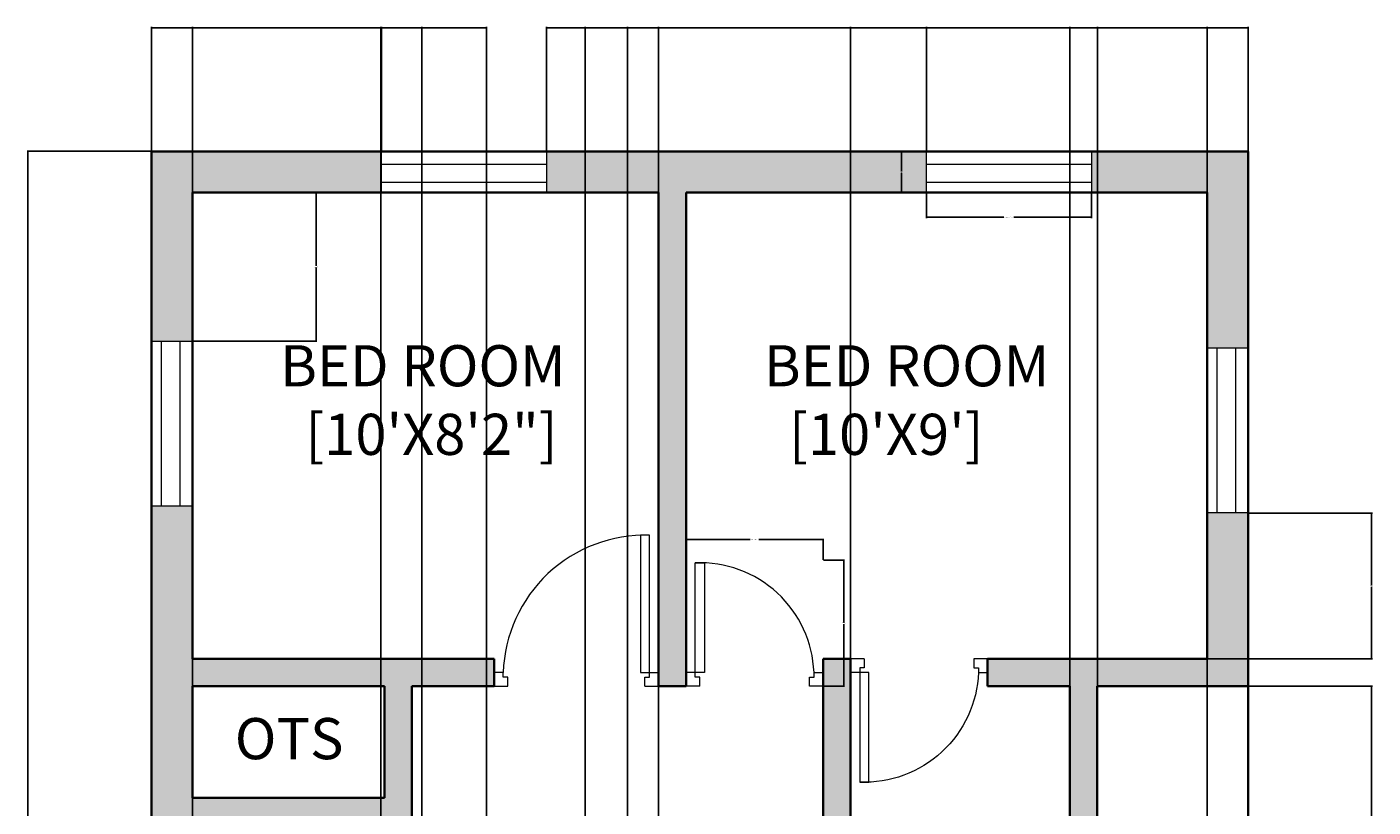
# Model space of a CAD drawing. Units: inches. Extents: x 1963 to 2258, y 1522 to 2116.
# Tile 3 of 3: x 1963 to 2257, y 1945 to 2116. Entities that reach past the tile are written whole.
import ezdxf

# ---------------------------------------------------------------- set-up
doc = ezdxf.new("R2010")
doc.units = ezdxf.units.IN
for name, color, linetype, lineweight in [('A-ANNO-DIMS', 2, 'Continuous', 18), ('A-AREA-IDEN', 7, 'Continuous', 18), ('A-DOOR', 3, 'Continuous', 18), ('A-GLAZ', 4, 'Continuous', 18), ('A-WALL', 7, 'Continuous', 35), ('A-WALL-PATT', 250, 'Continuous', 13)]:
    doc.layers.add(name, color=color, linetype=linetype, lineweight=lineweight)
doc.styles.get("Standard").update_dxf_attribs({"font": 'arial.ttf'})
doc.dimstyles.get("Standard").update_dxf_attribs({"dimtxt": 0.18, "dimasz": 0.18, "dimexe": 0.18, "dimexo": 0.0625, "dimgap": 0.09, "dimtad": 0, "dimtih": 1, "dimtoh": 1, "dimdec": 4, "dimzin": 0, "dimdsep": 46, "dimtxsty": 'Standard', "dimcen": 0.09, "dimadec": 0, "dimazin": 0, "dimtfac": 1, "dimtdec": 4, "dimtofl": 0, "dimtmove": 0, "dimatfit": 3, "dimfxl": 1, "dimtolj": 1, "dimtzin": 0, "dimarcsym": 0})

# ---------------------------------------------------------------- blocks, each defined once
blk = doc.blocks.new('WIN-36-9IN-WALL')
for p, q in [((-9, 0), (-9, 36.12)), ((-9, 36.12), (0, 36.12)), ((-6.81, 0), (-6.81, 36.12)), ((-4.5, 36.12), (-2.78, 36.12)), ((-2.78, 36.12), (-2.78, 0)), ((0, 36.12), (0, 0)), ((0, 0), (-9, 0)), ((-2.78, 0), (-6.81, 0)), ((0, 0), (-4.5, 0))]:
    blk.add_line(p, q)
blk = doc.blocks.new('DOOR-SWING-30IN')
for p, q in [((-3, -2), (-3, 0)), ((-3, 0), (0, 0)), ((-2, -2), (-3, -2)), ((-2, -3), (-2, -2)), ((0, 0), (0, -3)), ((0, 0), (0, -3)), ((0, -3), (-2, -3)), ((-27, -28), (-27, -26)), ((-27, -26), (-3, -26)), ((-3, -26), (-3, -28)), ((-3, -28), (-27, -28)), ((-2, -28), (-3, -28)), ((-3, -28), (-3, -30)), ((0, -27), (-2, -27)), ((-2, -27), (-2, -28)), ((0, -27), (0, -30)), ((-3, -30), (0, -30))]:
    blk.add_line(p, q)
blk.add_arc((-2, -27), 25.02, 92.2906, 182.2906)
blk = doc.blocks.new('DOOR-SWING-36IN')
for p, q in [((34, 33), (32, 33)), ((32, 33), (32, 3)), ((34, 3), (34, 33)), ((2, 3), (0, 3)), ((0, 3), (0, 0)), ((2, 2), (2, 3)), ((32, 3), (34, 3)), ((34, 2), (34, 3)), ((34, 3), (36, 3)), ((36, 3), (36, 0)), ((0, 0), (3, 0)), ((0, 0), (3, 0)), ((0, 0), (3, 0)), ((3, 2), (2, 2)), ((3, 0), (3, 2)), ((33, 0), (33, 2)), ((33, 2), (34, 2)), ((33, 0), (36, 0))]:
    blk.add_line(p, q)
blk.add_arc((33, 2), 31.02, 88.1524, 178.1524)
blk = doc.blocks.new('*D6')
at = {"layer": 'A-ANNO-DIMS', "color": 0, "lineweight": -2, "transparency": 16777216}
for p, q in [((2159.69, 2079.68), (2159.69, 2074.15)), ((2195.81, 2079.68), (2195.81, 2074.15)), ((2159.87, 2074.33), (2176.63, 2074.33)), ((2195.63, 2074.33), (2178.87, 2074.33))]:
    blk.add_line(p, q, dxfattribs=at)
at = {"layer": 'A-ANNO-DIMS', "color": 0, "transparency": 16777216}
for points in [[(2159.87, 2074.36), (2159.87, 2074.3), (2159.69, 2074.33)], [(2195.63, 2074.36), (2195.63, 2074.3), (2195.81, 2074.33)]]:
    blk.add_solid(points, dxfattribs=at)
at = {"layer": 'Defpoints', "color": 0, "transparency": 16777216}
for p in [(2159.69, 2079.75), (2195.81, 2079.75), (2159.69, 2074.33)]:
    blk.add_point(p, dxfattribs=at)
at = {"layer": 'A-ANNO-DIMS', "color": 0, "transparency": 16777216, "insert": (2177.75, 2074.33), "char_height": 0.18, "attachment_point": 5}
blk.add_mtext('\\A1;WINDOW 36 TYP.', dxfattribs=at)
blk = doc.blocks.new('*D7')
at = {"layer": 'A-ANNO-DIMS', "color": 0, "lineweight": -2, "transparency": 16777216}
for p, q in [((2159.63, 2088.75), (2154.09, 2088.75)), ((2154.27, 2088.57), (2154.27, 2084.43)), ((2154.27, 2079.93), (2154.27, 2084.07)), ((2159.63, 2079.75), (2154.09, 2079.75))]:
    blk.add_line(p, q, dxfattribs=at)
at = {"layer": 'A-ANNO-DIMS', "color": 0, "transparency": 16777216}
for points in [[(2154.24, 2088.57), (2154.3, 2088.57), (2154.27, 2088.75)], [(2154.24, 2079.93), (2154.3, 2079.93), (2154.27, 2079.75)]]:
    blk.add_solid(points, dxfattribs=at)
at = {"layer": 'Defpoints', "color": 0, "transparency": 16777216}
for p in [(2154.27, 2088.75), (2159.69, 2088.75), (2159.69, 2079.75)]:
    blk.add_point(p, dxfattribs=at)
at = {"layer": 'A-ANNO-DIMS', "color": 0, "transparency": 16777216, "insert": (2154.27, 2084.25), "char_height": 0.18, "attachment_point": 5}
blk.add_mtext('\\A1;9 TYP.', dxfattribs=at)
blk = doc.blocks.new('*D10')
at = {"layer": 'A-ANNO-DIMS', "color": 0, "lineweight": -2, "transparency": 16777216}
for p, q in [((2107.11, 1999.36), (2107.11, 2003.98)), ((2107.29, 2003.8), (2121.17, 2003.8)), ((2136.93, 2003.8), (2123.04, 2003.8)), ((2137.11, 1999.36), (2137.11, 2003.98))]:
    blk.add_line(p, q, dxfattribs=at)
at = {"layer": 'A-ANNO-DIMS', "color": 0, "transparency": 16777216}
for points in [[(2107.29, 2003.83), (2107.29, 2003.77), (2107.11, 2003.8)], [(2136.93, 2003.83), (2136.93, 2003.77), (2137.11, 2003.8)]]:
    blk.add_solid(points, dxfattribs=at)
at = {"layer": 'Defpoints', "color": 0, "transparency": 16777216}
for p in [(2137.11, 2003.8), (2107.11, 1999.3), (2137.11, 1999.3)]:
    blk.add_point(p, dxfattribs=at)
at = {"layer": 'A-ANNO-DIMS', "color": 0, "transparency": 16777216, "insert": (2122.11, 2003.8), "char_height": 0.18, "attachment_point": 5}
blk.add_mtext('\\A1;DOOR 30 TYP.', dxfattribs=at)
blk = doc.blocks.new('*D11')
at = {"layer": 'A-ANNO-DIMS', "color": 0, "lineweight": -2, "transparency": 16777216}
for p, q in [((2137.17, 1999.3), (2141.79, 1999.3)), ((2141.61, 1999.12), (2141.61, 1985.71)), ((2141.61, 1971.93), (2141.61, 1985.34)), ((2137.17, 1971.75), (2141.79, 1971.75))]:
    blk.add_line(p, q, dxfattribs=at)
at = {"layer": 'A-ANNO-DIMS', "color": 0, "transparency": 16777216}
for points in [[(2141.58, 1999.12), (2141.64, 1999.12), (2141.61, 1999.3)], [(2141.58, 1971.93), (2141.64, 1971.93), (2141.61, 1971.75)]]:
    blk.add_solid(points, dxfattribs=at)
at = {"layer": 'Defpoints', "color": 0, "transparency": 16777216}
for p in [(2137.11, 1999.3), (2137.11, 1971.75), (2141.61, 1971.75)]:
    blk.add_point(p, dxfattribs=at)
at = {"layer": 'A-ANNO-DIMS', "color": 0, "transparency": 16777216, "insert": (2141.61, 1985.52), "char_height": 0.18, "attachment_point": 5}
blk.add_mtext('\\A1;28 TYP.', dxfattribs=at)
blk = doc.blocks.new('*D15')
at = {"layer": 'A-ANNO-DIMS', "color": 0, "lineweight": -2, "transparency": 16777216}
for p, q in [((2094.32, 1548.81), (2094.32, 2115.96)), ((2094.5, 2115.78), (2157.26, 2115.78)), ((2220.93, 2115.78), (2158.17, 2115.78)), ((2221.11, 1548.81), (2221.11, 2115.96))]:
    blk.add_line(p, q, dxfattribs=at)
at = {"layer": 'A-ANNO-DIMS', "color": 0, "transparency": 16777216}
for points in [[(2094.5, 2115.81), (2094.5, 2115.75), (2094.32, 2115.78)], [(2220.93, 2115.81), (2220.93, 2115.75), (2221.11, 2115.78)]]:
    blk.add_solid(points, dxfattribs=at)
at = {"layer": 'Defpoints', "color": 0, "transparency": 16777216}
for p in [(2221.11, 2115.78), (2094.32, 1548.75), (2221.11, 1548.75)]:
    blk.add_point(p, dxfattribs=at)
at = {"layer": 'A-ANNO-DIMS', "color": 0, "transparency": 16777216, "insert": (2157.72, 2115.78), "char_height": 0.18, "attachment_point": 5}
blk.add_mtext('\\A1;126.79', dxfattribs=at)
blk = doc.blocks.new('*D16')
at = {"layer": 'A-ANNO-DIMS', "color": 0, "lineweight": -2, "transparency": 16777216}
for p, q in [((1990.11, 2088.81), (1990.11, 2115.96)), ((1990.29, 2115.78), (2014.88, 2115.78)), ((2040.25, 2115.78), (2015.66, 2115.78)), ((2040.43, 2088.81), (2040.43, 2115.96))]:
    blk.add_line(p, q, dxfattribs=at)
at = {"layer": 'A-ANNO-DIMS', "color": 0, "transparency": 16777216}
for points in [[(1990.29, 2115.81), (1990.29, 2115.75), (1990.11, 2115.78)], [(2040.25, 2115.81), (2040.25, 2115.75), (2040.43, 2115.78)]]:
    blk.add_solid(points, dxfattribs=at)
at = {"layer": 'Defpoints', "color": 0, "transparency": 16777216}
for p in [(2040.43, 2115.78), (1990.11, 2088.75), (2040.43, 2088.75)]:
    blk.add_point(p, dxfattribs=at)
at = {"layer": 'A-ANNO-DIMS', "color": 0, "transparency": 16777216, "insert": (2015.27, 2115.78), "char_height": 0.18, "attachment_point": 5}
blk.add_mtext('\\A1;50.32', dxfattribs=at)
blk = doc.blocks.new('*D17')
at = {"layer": 'A-ANNO-DIMS', "color": 0, "lineweight": -2, "transparency": 16777216}
for p, q in [((2076.55, 2088.81), (2076.55, 2115.96)), ((2076.73, 2115.78), (2117.73, 2115.78)), ((2159.51, 2115.78), (2118.51, 2115.78)), ((2159.69, 2088.81), (2159.69, 2115.96))]:
    blk.add_line(p, q, dxfattribs=at)
at = {"layer": 'A-ANNO-DIMS', "color": 0, "transparency": 16777216}
for points in [[(2076.73, 2115.81), (2076.73, 2115.75), (2076.55, 2115.78)], [(2159.51, 2115.81), (2159.51, 2115.75), (2159.69, 2115.78)]]:
    blk.add_solid(points, dxfattribs=at)
at = {"layer": 'Defpoints', "color": 0, "transparency": 16777216}
for p in [(2159.69, 2115.78), (2076.55, 2088.75), (2159.69, 2088.75)]:
    blk.add_point(p, dxfattribs=at)
at = {"layer": 'A-ANNO-DIMS', "color": 0, "transparency": 16777216, "insert": (2118.12, 2115.78), "char_height": 0.18, "attachment_point": 5}
blk.add_mtext('\\A1;83.14', dxfattribs=at)
blk = doc.blocks.new('*D18')
at = {"layer": 'A-ANNO-DIMS', "color": 0, "lineweight": -2, "transparency": 16777216}
for p, q in [((1999.11, 2079.68), (1999.11, 1521.53)), ((2101.11, 2079.68), (2101.11, 1521.53)), ((1999.29, 1521.71), (2049.83, 1521.71)), ((2100.93, 1521.71), (2050.39, 1521.71))]:
    blk.add_line(p, q, dxfattribs=at)
at = {"layer": 'A-ANNO-DIMS', "color": 0, "transparency": 16777216}
for points in [[(1999.29, 1521.74), (1999.29, 1521.68), (1999.11, 1521.71)], [(2100.93, 1521.74), (2100.93, 1521.68), (2101.11, 1521.71)]]:
    blk.add_solid(points, dxfattribs=at)
at = {"layer": 'Defpoints', "color": 0, "transparency": 16777216}
for p in [(1999.11, 2079.75), (2101.11, 2079.75), (2101.11, 1521.71)]:
    blk.add_point(p, dxfattribs=at)
at = {"layer": 'A-ANNO-DIMS', "color": 0, "transparency": 16777216, "insert": (2050.11, 1521.71), "char_height": 0.18, "attachment_point": 5}
blk.add_mtext('\\A1;102', dxfattribs=at)
blk = doc.blocks.new('*D25')
at = {"layer": 'A-ANNO-DIMS', "color": 0, "lineweight": -2, "transparency": 16777216}
for p, q in [((1999.17, 2079.75), (2026.32, 2079.75)), ((2026.14, 2079.57), (2026.14, 2063.67)), ((2026.14, 2047.42), (2026.14, 2063.31)), ((1999.17, 2047.24), (2026.32, 2047.24))]:
    blk.add_line(p, q, dxfattribs=at)
at = {"layer": 'A-ANNO-DIMS', "color": 0, "transparency": 16777216}
for points in [[(2026.11, 2079.57), (2026.17, 2079.57), (2026.14, 2079.75)], [(2026.11, 2047.42), (2026.17, 2047.42), (2026.14, 2047.24)]]:
    blk.add_solid(points, dxfattribs=at)
at = {"layer": 'Defpoints', "color": 0, "transparency": 16777216}
for p in [(1999.11, 2079.75), (1999.11, 2047.24), (2026.14, 2047.24)]:
    blk.add_point(p, dxfattribs=at)
at = {"layer": 'A-ANNO-DIMS', "color": 0, "transparency": 16777216, "insert": (2026.14, 2063.49), "char_height": 0.18, "attachment_point": 5}
blk.add_mtext('\\A1;32.51', dxfattribs=at)
blk = doc.blocks.new('*D29')
at = {"layer": 'A-ANNO-DIMS', "color": 0, "lineweight": -2, "transparency": 16777216}
for p, q in [((2230.17, 1971.75), (2257.32, 1971.75)), ((2257.14, 1971.57), (2257.14, 1934.43)), ((2257.14, 1896.93), (2257.14, 1934.07)), ((2221.17, 1896.75), (2257.32, 1896.75))]:
    blk.add_line(p, q, dxfattribs=at)
at = {"layer": 'A-ANNO-DIMS', "color": 0, "transparency": 16777216}
for points in [[(2257.11, 1971.57), (2257.17, 1971.57), (2257.14, 1971.75)], [(2257.11, 1896.93), (2257.17, 1896.93), (2257.14, 1896.75)]]:
    blk.add_solid(points, dxfattribs=at)
at = {"layer": 'Defpoints', "color": 0, "transparency": 16777216}
for p in [(2230.11, 1971.75), (2257.14, 1971.75), (2221.11, 1896.75)]:
    blk.add_point(p, dxfattribs=at)
at = {"layer": 'A-ANNO-DIMS', "color": 0, "transparency": 16777216, "insert": (2257.14, 1934.25), "char_height": 0.18, "attachment_point": 5}
blk.add_mtext('\\A1;75', dxfattribs=at)
blk = doc.blocks.new('*D32')
at = {"layer": 'A-ANNO-DIMS', "color": 0, "lineweight": -2, "transparency": 16777216}
for p, q in [((2230.17, 2009.63), (2257.32, 2009.63)), ((2257.14, 2009.45), (2257.14, 1993.87)), ((2257.14, 1977.93), (2257.14, 1993.51)), ((2221.17, 1977.75), (2257.32, 1977.75))]:
    blk.add_line(p, q, dxfattribs=at)
at = {"layer": 'A-ANNO-DIMS', "color": 0, "transparency": 16777216}
for points in [[(2257.11, 2009.45), (2257.17, 2009.45), (2257.14, 2009.63)], [(2257.11, 1977.93), (2257.17, 1977.93), (2257.14, 1977.75)]]:
    blk.add_solid(points, dxfattribs=at)
at = {"layer": 'Defpoints', "color": 0, "transparency": 16777216}
for p in [(2230.11, 2009.63), (2221.11, 1977.75), (2257.14, 1977.75)]:
    blk.add_point(p, dxfattribs=at)
at = {"layer": 'A-ANNO-DIMS', "color": 0, "transparency": 16777216, "insert": (2257.14, 1993.69), "char_height": 0.18, "attachment_point": 5}
blk.add_mtext('\\A1;31.89', dxfattribs=at)
blk = doc.blocks.new('*D34')
at = {"layer": 'A-ANNO-DIMS', "color": 0, "lineweight": -2, "transparency": 16777216}
for p, q in [((2047.11, 1971.68), (2047.11, 1521.53)), ((2137.11, 1971.68), (2137.11, 1521.53)), ((2047.29, 1521.71), (2091.89, 1521.71)), ((2136.93, 1521.71), (2092.33, 1521.71))]:
    blk.add_line(p, q, dxfattribs=at)
at = {"layer": 'A-ANNO-DIMS', "color": 0, "transparency": 16777216}
for points in [[(2047.29, 1521.74), (2047.29, 1521.68), (2047.11, 1521.71)], [(2136.93, 1521.74), (2136.93, 1521.68), (2137.11, 1521.71)]]:
    blk.add_solid(points, dxfattribs=at)
at = {"layer": 'Defpoints', "color": 0, "transparency": 16777216}
for p in [(2047.11, 1971.75), (2137.11, 1971.75), (2137.11, 1521.71)]:
    blk.add_point(p, dxfattribs=at)
at = {"layer": 'A-ANNO-DIMS', "color": 0, "transparency": 16777216, "insert": (2092.11, 1521.71), "char_height": 0.18, "attachment_point": 5}
blk.add_mtext('\\A1;90', dxfattribs=at)
blk = doc.blocks.new('*D35')
at = {"layer": 'A-ANNO-DIMS', "color": 0, "lineweight": -2, "transparency": 16777216}
for p, q in [((2197.11, 1902.81), (2197.11, 2115.96)), ((2197.29, 2115.78), (2213.39, 2115.78)), ((2229.93, 2115.78), (2213.83, 2115.78)), ((2230.11, 1902.81), (2230.11, 2115.96))]:
    blk.add_line(p, q, dxfattribs=at)
at = {"layer": 'A-ANNO-DIMS', "color": 0, "transparency": 16777216}
for points in [[(2197.29, 2115.81), (2197.29, 2115.75), (2197.11, 2115.78)], [(2229.93, 2115.81), (2229.93, 2115.75), (2230.11, 2115.78)]]:
    blk.add_solid(points, dxfattribs=at)
at = {"layer": 'Defpoints', "color": 0, "transparency": 16777216}
for p in [(2230.11, 2115.78), (2197.11, 1902.75), (2230.11, 1902.75)]:
    blk.add_point(p, dxfattribs=at)
at = {"layer": 'A-ANNO-DIMS', "color": 0, "transparency": 16777216, "insert": (2213.61, 2115.78), "char_height": 0.18, "attachment_point": 5}
blk.add_mtext('\\A1;33', dxfattribs=at)
blk = doc.blocks.new('*D36')
at = {"layer": 'A-ANNO-DIMS', "color": 0, "lineweight": -2, "transparency": 16777216}
for p, q in [((2143.11, 1902.81), (2143.11, 2115.96)), ((2143.29, 2115.78), (2166.89, 2115.78)), ((2190.93, 2115.78), (2167.33, 2115.78)), ((2191.11, 1902.81), (2191.11, 2115.96))]:
    blk.add_line(p, q, dxfattribs=at)
at = {"layer": 'A-ANNO-DIMS', "color": 0, "transparency": 16777216}
for points in [[(2143.29, 2115.81), (2143.29, 2115.75), (2143.11, 2115.78)], [(2190.93, 2115.81), (2190.93, 2115.75), (2191.11, 2115.78)]]:
    blk.add_solid(points, dxfattribs=at)
at = {"layer": 'Defpoints', "color": 0, "transparency": 16777216}
for p in [(2143.11, 2115.78), (2143.11, 1902.75), (2191.11, 1902.75)]:
    blk.add_point(p, dxfattribs=at)
at = {"layer": 'A-ANNO-DIMS', "color": 0, "transparency": 16777216, "insert": (2167.11, 2115.78), "char_height": 0.18, "attachment_point": 5}
blk.add_mtext('\\A1;48', dxfattribs=at)
blk = doc.blocks.new('*D37')
at = {"layer": 'A-ANNO-DIMS', "color": 0, "lineweight": -2, "transparency": 16777216}
for p, q in [((1999.11, 1743.38), (1999.11, 2115.96)), ((1999.29, 2115.78), (2030.89, 2115.78)), ((2063.27, 2115.78), (2031.67, 2115.78)), ((2063.45, 1743.38), (2063.45, 2115.96))]:
    blk.add_line(p, q, dxfattribs=at)
at = {"layer": 'A-ANNO-DIMS', "color": 0, "transparency": 16777216}
for points in [[(1999.29, 2115.81), (1999.29, 2115.75), (1999.11, 2115.78)], [(2063.27, 2115.81), (2063.27, 2115.75), (2063.45, 2115.78)]]:
    blk.add_solid(points, dxfattribs=at)
at = {"layer": 'Defpoints', "color": 0, "transparency": 16777216}
for p in [(2063.45, 2115.78), (1999.11, 1743.32), (2063.45, 1743.32)]:
    blk.add_point(p, dxfattribs=at)
at = {"layer": 'A-ANNO-DIMS', "color": 0, "transparency": 16777216, "insert": (2031.28, 2115.78), "char_height": 0.18, "attachment_point": 5}
blk.add_mtext('\\A1;64.34', dxfattribs=at)
blk = doc.blocks.new('*D38')
at = {"layer": 'A-ANNO-DIMS', "color": 0, "lineweight": -2, "transparency": 16777216}
for p, q in [((1999.11, 1647.38), (1999.11, 2115.96)), ((1999.29, 2115.78), (2023.84, 2115.78)), ((2049.14, 2115.78), (2024.59, 2115.78)), ((2049.32, 1647.35), (2049.32, 2115.96))]:
    blk.add_line(p, q, dxfattribs=at)
at = {"layer": 'A-ANNO-DIMS', "color": 0, "transparency": 16777216}
for points in [[(1999.29, 2115.81), (1999.29, 2115.75), (1999.11, 2115.78)], [(2049.14, 2115.81), (2049.14, 2115.75), (2049.32, 2115.78)]]:
    blk.add_solid(points, dxfattribs=at)
at = {"layer": 'Defpoints', "color": 0, "transparency": 16777216}
for p in [(2049.32, 2115.78), (1999.11, 1647.32), (2049.32, 1647.29)]:
    blk.add_point(p, dxfattribs=at)
at = {"layer": 'A-ANNO-DIMS', "color": 0, "transparency": 16777216, "insert": (2024.22, 2115.78), "char_height": 0.18, "attachment_point": 5}
blk.add_mtext('\\A1;50.21', dxfattribs=at)
blk = doc.blocks.new('*D42')
at = {"layer": 'A-ANNO-DIMS', "color": 0, "lineweight": -2, "transparency": 16777216}
for p, q in [((1999.11, 1557.81), (1999.11, 2115.96)), ((1999.29, 2115.78), (2019.25, 2115.78)), ((2040.14, 2115.78), (2020.18, 2115.78)), ((2040.32, 1557.81), (2040.32, 2115.96))]:
    blk.add_line(p, q, dxfattribs=at)
at = {"layer": 'A-ANNO-DIMS', "color": 0, "transparency": 16777216}
for points in [[(1999.29, 2115.81), (1999.29, 2115.75), (1999.11, 2115.78)], [(2040.14, 2115.81), (2040.14, 2115.75), (2040.32, 2115.78)]]:
    blk.add_solid(points, dxfattribs=at)
at = {"layer": 'Defpoints', "color": 0, "transparency": 16777216}
for p in [(2040.32, 2115.78), (1999.11, 1557.75), (2040.32, 1557.75)]:
    blk.add_point(p, dxfattribs=at)
at = {"layer": 'A-ANNO-DIMS', "color": 0, "transparency": 16777216, "insert": (2019.72, 2115.78), "char_height": 0.18, "attachment_point": 5}
blk.add_mtext('\\A1;41.214', dxfattribs=at)
blk = doc.blocks.new('*D43')
at = {"layer": 'A-ANNO-DIMS', "color": 0, "lineweight": -2, "transparency": 16777216}
for p, q in [((2040.32, 1557.81), (2040.32, 2115.96)), ((2040.5, 2115.78), (2044.67, 2115.78)), ((2049.14, 2115.78), (2044.97, 2115.78)), ((2049.32, 1557.81), (2049.32, 2115.96))]:
    blk.add_line(p, q, dxfattribs=at)
at = {"layer": 'A-ANNO-DIMS', "color": 0, "transparency": 16777216}
for points in [[(2040.5, 2115.81), (2040.5, 2115.75), (2040.32, 2115.78)], [(2049.14, 2115.81), (2049.14, 2115.75), (2049.32, 2115.78)]]:
    blk.add_solid(points, dxfattribs=at)
at = {"layer": 'Defpoints', "color": 0, "transparency": 16777216}
for p in [(2049.32, 2115.78), (2040.32, 1557.75), (2049.32, 1557.75)]:
    blk.add_point(p, dxfattribs=at)
at = {"layer": 'A-ANNO-DIMS', "color": 0, "transparency": 16777216, "insert": (2044.82, 2115.78), "char_height": 0.18, "attachment_point": 5}
blk.add_mtext('\\A1;9', dxfattribs=at)
blk = doc.blocks.new('*D46')
at = {"layer": 'A-ANNO-DIMS', "color": 0, "lineweight": -2, "transparency": 16777216}
for p, q in [((2085.06, 1647.35), (2085.06, 2115.96)), ((2085.24, 2115.78), (2092.7, 2115.78)), ((2100.93, 2115.78), (2093.47, 2115.78)), ((2101.11, 1647.38), (2101.11, 2115.96))]:
    blk.add_line(p, q, dxfattribs=at)
at = {"layer": 'A-ANNO-DIMS', "color": 0, "transparency": 16777216}
for points in [[(2085.24, 2115.81), (2085.24, 2115.75), (2085.06, 2115.78)], [(2100.93, 2115.81), (2100.93, 2115.75), (2101.11, 2115.78)]]:
    blk.add_solid(points, dxfattribs=at)
at = {"layer": 'Defpoints', "color": 0, "transparency": 16777216}
for p in [(2101.11, 2115.78), (2085.06, 1647.29), (2101.11, 1647.32)]:
    blk.add_point(p, dxfattribs=at)
at = {"layer": 'A-ANNO-DIMS', "color": 0, "transparency": 16777216, "insert": (2093.08, 2115.78), "char_height": 0.18, "attachment_point": 5}
blk.add_mtext('\\A1;16.05', dxfattribs=at)
blk = doc.blocks.new('*D47')
at = {"layer": 'A-ANNO-DIMS', "color": 0, "lineweight": -2, "transparency": 16777216}
for p, q in [((1990.05, 2088.75), (1962.89, 2088.75)), ((1963.07, 2088.57), (1963.07, 1818.93)), ((1963.07, 1548.93), (1963.07, 1818.57)), ((1990.05, 1548.75), (1962.89, 1548.75))]:
    blk.add_line(p, q, dxfattribs=at)
at = {"layer": 'A-ANNO-DIMS', "color": 0, "transparency": 16777216}
for points in [[(1963.04, 2088.57), (1963.1, 2088.57), (1963.07, 2088.75)], [(1963.04, 1548.93), (1963.1, 1548.93), (1963.07, 1548.75)]]:
    blk.add_solid(points, dxfattribs=at)
at = {"layer": 'Defpoints', "color": 0, "transparency": 16777216}
for p in [(1963.07, 2088.75), (1990.11, 2088.75), (1990.11, 1548.75)]:
    blk.add_point(p, dxfattribs=at)
at = {"layer": 'A-ANNO-DIMS', "color": 0, "transparency": 16777216, "insert": (1963.07, 1818.75), "char_height": 0.18, "attachment_point": 5}
blk.add_mtext('\\A1;540', dxfattribs=at)

msp = doc.modelspace()

# ---------------------------------------------------------------- hatches: boundary and pattern name
at = {"layer": 'A-WALL-PATT'}
h = msp.add_hatch(color=256, dxfattribs=at)
h.dxf.hatch_style = 1
h.paths.add_polyline_path([(2040.4282, 2088.7475), (1990.109, 2088.7475), (1990.109, 2047.2372), (1999.109, 2047.2372), (1999.109, 2079.7475), (2040.4282, 2079.7475)])
h.paths.add_polyline_path([(2159.691, 2088.7475), (2076.5488, 2088.7475), (2076.5488, 2084.2475), (2076.5488, 2079.7475), (2101.109, 2079.7475), (2101.109, 1977.7475), (2101.109, 1971.7475), (2107.109, 1971.7475), (2107.109, 1974.7475), (2107.109, 1977.7475), (2107.109, 2079.7475), (2110.109, 2079.7475), (2159.691, 2079.7475)])
h.paths.add_polyline_path([(2230.109, 2088.7475), (2195.8116, 2088.7475), (2195.8116, 2084.2475), (2195.8116, 2079.7475), (2221.109, 2079.7475), (2221.109, 2045.7556), (2230.109, 2045.7556)])
h.paths.add_polyline_path([(2230.109, 2009.6349), (2225.609, 2009.6349), (2221.109, 2009.6349), (2221.109, 1977.7475), (2173.109, 1977.7475), (2173.109, 1974.7475), (2173.0802, 1971.7475), (2178.9852, 1971.7475), (2185.109, 1971.7475), (2191.109, 1971.7475), (2191.109, 1902.7475), (2143.109, 1902.7475), (2143.109, 1971.7475), (2143.109, 1977.7475), (2137.109, 1977.7475), (2137.109, 1971.7475), (2137.109, 1902.7475), (2101.109, 1902.7475), (2101.109, 1830.7475), (2104.109, 1830.7475), (2107.109, 1830.7475), (2107.109, 1896.7475), (2221.109, 1896.7475), (2221.109, 1871.2465), (2230.109, 1871.2465), (2230.109, 1902.7475), (2197.109, 1902.7475), (2197.109, 1971.7475), (2230.109, 1971.7475)])
h.paths.add_polyline_path([(2065.109, 1977.7475), (1999.109, 1977.7475), (1999.109, 2011.1166), (1994.609, 2011.1166), (1990.109, 2011.1166), (1990.109, 1810.0744), (1999.109, 1810.0744), (1999.109, 1863.32), (2047.109, 1863.32), (2047.109, 1869.32), (2047.109, 1911.4119), (2044.109, 1911.4119), (2041.109, 1911.4119), (2041.109, 1869.32), (1999.109, 1869.32), (1999.109, 1941.32), (2041.109, 1941.32), (2044.109, 1941.32), (2044.109, 1941.4119), (2047.109, 1941.4119), (2047.109, 1971.7475), (2065.109, 1971.7475), (2065.109, 1974.7475)])
h.paths.add_polyline_path([(2041.109, 1971.7475), (2041.109, 1947.32), (1999.109, 1947.32), (1999.109, 1971.7475)], flags=16)
h.paths.add_polyline_path([(2230.109, 1835.1259), (2225.609, 1835.1259), (2221.109, 1835.1259), (2221.109, 1794.7475), (2101.109, 1794.7475), (2101.109, 1788.7475), (2221.109, 1788.7475), (2221.109, 1763.2023), (2230.109, 1763.2023)])
h.paths.add_polyline_path([(2063.4524, 1743.32), (1999.109, 1743.32), (1999.109, 1773.9538), (1994.609, 1773.9538), (1992.3007, 1773.9538), (1990.109, 1773.9538), (1990.109, 1703.9859), (1999.109, 1703.9859), (1999.109, 1737.32), (2063.4524, 1737.32)])
h.paths.add_polyline_path([(2169.7564, 1696.9689), (2169.7564, 1698.7475), (2143.109, 1698.7475), (2143.109, 1692.7475), (2143.6022, 1692.7475), (2169.7564, 1692.7475), (2169.7564, 1695.7336)])
h.paths.add_polyline_path([(2230.109, 1727.0817), (2225.609, 1727.0817), (2221.109, 1727.0817), (2221.109, 1698.7475), (2205.4934, 1698.7475), (2205.4934, 1692.7475), (2221.109, 1692.7475), (2221.109, 1557.7475), (2221.109, 1548.7475), (2230.109, 1548.7475)])
h.paths.add_polyline_path([(2107.109, 1760.0903), (2101.109, 1760.0903), (2101.109, 1743.32), (2101.109, 1737.32), (2101.109, 1698.7475), (2101.109, 1687.7398), (2104.1229, 1687.7398), (2105.3583, 1687.7398), (2107.109, 1687.7398), (2107.109, 1692.7475), (2107.109, 1695.7475), (2107.109, 1698.7475)])
h.paths.add_polyline_path([(2107.109, 1652.0028), (2101.109, 1652.0028), (2101.109, 1647.32), (2085.0601, 1647.32), (2085.0601, 1641.32), (2085.3232, 1641.32), (2107.109, 1641.32)])
h.paths.add_polyline_path([(2049.3232, 1645.5414), (2049.3232, 1647.32), (1999.109, 1647.32), (1999.109, 1667.8653), (1994.609, 1667.8653), (1992.3007, 1667.8653), (1990.109, 1667.8653), (1990.109, 1548.7475), (2094.3232, 1548.7475), (2094.3232, 1557.7475), (2085.3232, 1557.7475), (1999.109, 1557.7475), (1999.109, 1641.32), (2049.3232, 1641.32), (2049.3232, 1644.306)])

# ---------------------------------------------------------------- linework, layer by layer
at = {"layer": 'A-WALL'}
for p, q in [((1999.109, 2079.7475), (2101.109, 2079.7475)), ((1999.109, 2079.7475), (1999.109, 1981.7475)), ((2101.109, 1977.7475), (2101.109, 2079.7475)), ((2107.109, 1977.7475), (2107.109, 2079.7475)), ((2107.109, 2079.7475), (2110.109, 2079.7475)), ((2221.109, 2079.7475), (2221.109, 1977.7475)), ((2065.109, 1977.7475), (1999.109, 1977.7475)), ((2065.109, 1971.7475), (2065.109, 1977.7475)), ((2101.109, 1977.7475), (2101.109, 1971.7475)), ((2107.109, 1971.7475), (2107.109, 1977.7475)), ((2137.109, 1971.7475), (2137.109, 1977.7475)), ((2143.109, 1977.7475), (2137.109, 1977.7475)), ((2143.109, 1971.7475), (2143.109, 1977.7475)), ((2143.109, 1971.7475), (2143.109, 1977.7475)), ((2221.109, 1977.7475), (2173.0802, 1977.7475)), ((2173.0802, 1977.7475), (2173.0802, 1971.7475)), ((2041.109, 1971.7475), (1999.109, 1971.7475)), ((2041.109, 1947.32), (2041.109, 1971.7475)), ((2047.109, 1941.32), (2047.109, 1971.7475)), ((2065.109, 1971.7475), (2047.109, 1971.7475)), ((2107.109, 1971.7475), (2101.109, 1971.7475)), ((2101.109, 1971.7475), (2107.109, 1971.7475)), ((2137.109, 1902.7475), (2137.109, 1971.7475)), ((2143.109, 1902.7475), (2143.109, 1971.7475)), ((2173.0802, 1971.7475), (2178.9852, 1971.7475)), ((2178.9852, 1971.7475), (2173.0802, 1971.7475)), ((2185.109, 1971.7475), (2178.9852, 1971.7475)), ((2191.109, 1971.7475), (2184.9852, 1971.7475)), ((2191.109, 1902.7475), (2191.109, 1971.7475)), ((2230.109, 1971.7475), (2197.109, 1971.7475)), ((2197.109, 1902.7475), (2197.109, 1971.7475)), ((2041.109, 1947.32), (1999.109, 1947.32))]:
    msp.add_line(p, q, dxfattribs=at)
for points in [[(1990.109, 2088.7475), (2230.109, 2088.7475), (2230.109, 1548.7475), (1990.109, 1548.7475), (1990.109, 2088.7475)], [(1999.109, 1977.7475), (1999.109, 2079.7475), (2101.109, 2079.7475)], [(2107.109, 2079.7475), (2221.109, 2079.7475), (2221.109, 1977.7475)], [(1999.109, 1947.32), (1999.109, 1971.7475)]]:
    msp.add_lwpolyline(points, dxfattribs=at)

# ---------------------------------------------------------------- block references
at = {"layer": 'A-DOOR'}
msp.add_blockref('DOOR-SWING-36IN', (2065.109, 1971.7475), dxfattribs=at)
at = {"layer": 'A-DOOR', "rotation": 270.0000000000029}
msp.add_blockref('DOOR-SWING-30IN', (2137.109, 1971.7475), dxfattribs=at)
at = {"layer": 'A-DOOR', "extrusion": (0, 0, -1), "zscale": -1, "rotation": 89.99999999999999}
msp.add_blockref('DOOR-SWING-30IN', (-2173.109, 1977.7475), dxfattribs=at)
at = {"layer": 'A-GLAZ'}
for p, rotation in [((2076.5488, 2088.7475), 90.00000000000003), ((2195.8116, 2088.7475), 89.99999999999898)]:
    msp.add_blockref('WIN-36-9IN-WALL', p, dxfattribs=dict(at, rotation=rotation))
for p in [(1999.109, 2011.1166), (2230.109, 2009.6349)]:
    msp.add_blockref('WIN-36-9IN-WALL', p, dxfattribs=at)

# ---------------------------------------------------------------- texts
at = {"layer": 'A-AREA-IDEN', "char_height": 9, "attachment_point": 1}
for s, width, heights, insert in [('BED ROOM\\P  [10\'X8\'2"]', 109.520674, [52.7189], (2018.2756, 2046.3432)), ("BED ROOM\\P  [10'X9']", 109.520674, [52.7189], (2124.1291, 2046.3432)), ('OTS', 32.745855, [0], (2008.3632, 1964.7741))]:
    msp.add_mtext_dynamic_manual_height_columns(s, width=width, gutter_width=12.5, heights=heights, dxfattribs=dict(at, insert=insert))

# ---------------------------------------------------------------- dimensions: what is measured, and where the dimension line sits
at = {"layer": 'A-ANNO-DIMS'}
for base, p1, p2, override, picture, middle in [((2040.4282, 2115.7825), (1990.109, 2088.7475), (2040.4282, 2088.7475), {"dimdec": 2, "dimlfac": 1, "dimrnd": 0, "dimzin": 0, "dimdsep": 46, "dimlunit": 2}, '*D16', (2015.2686, 2115.7825)), ((2063.4524, 2115.7825), (1999.109, 1743.32), (2063.4524, 1743.32), {"dimdec": 2, "dimlfac": 1, "dimrnd": 0, "dimzin": 0, "dimdsep": 46, "dimlunit": 2}, '*D37', (2031.2807, 2115.7825)), ((2049.3232, 2115.7825), (1999.109, 1647.32), (2049.3232, 1647.2921), {"dimdec": 2, "dimlfac": 1, "dimrnd": 0, "dimzin": 0, "dimdsep": 46, "dimlunit": 2}, '*D38', (2024.2161, 2115.7825)), ((2040.3232, 2115.7825), (1999.109, 1557.7475), (2040.3232, 1557.7475), {"dimdec": 3, "dimlfac": 1, "dimrnd": 0, "dimzin": 0, "dimdsep": 46, "dimlunit": 2}, '*D42', (2019.7161, 2115.7825)), ((2049.3232, 2115.7825), (2040.3232, 1557.7475), (2049.3232, 1557.7475), {"dimdec": 0, "dimlfac": 1, "dimrnd": 0, "dimzin": 0, "dimdsep": 46, "dimlunit": 2}, '*D43', (2044.8232, 2115.7825)), ((2159.691, 2115.7825), (2076.5488, 2088.7475), (2159.691, 2088.7475), {"dimdec": 2, "dimlfac": 1, "dimrnd": 0, "dimzin": 0, "dimdsep": 46, "dimlunit": 2}, '*D17', (2118.1199, 2115.7825)), ((2101.109, 2115.7825), (2085.0601, 1647.2921), (2101.109, 1647.32), {"dimdec": 2, "dimlfac": 1, "dimrnd": 0, "dimzin": 0, "dimdsep": 46, "dimlunit": 2}, '*D46', (2093.0846, 2115.7825)), ((2221.109, 2115.7825), (2094.3232, 1548.7475), (2221.109, 1548.7475), {"dimdec": 2, "dimlfac": 1, "dimrnd": 0, "dimzin": 0, "dimdsep": 46, "dimlunit": 2}, '*D15', (2157.7161, 2115.7825)), ((2143.109, 2115.7825), (2191.109, 1902.7475), (2143.109, 1902.7475), {"dimdec": 0, "dimlfac": 1, "dimrnd": 0, "dimzin": 0, "dimdsep": 46, "dimlunit": 2}, '*D36', (2167.109, 2115.7825)), ((2230.109, 2115.7825), (2197.109, 1902.7475), (2230.109, 1902.7475), {"dimdec": 0, "dimlfac": 1, "dimrnd": 0, "dimzin": 0, "dimdsep": 46, "dimlunit": 2}, '*D35', (2213.609, 2115.7825)), ((2101.109, 1521.7125), (1999.109, 2079.7475), (2101.109, 2079.7475), {"dimdec": 0, "dimlfac": 1, "dimrnd": 0, "dimzin": 0, "dimdsep": 46, "dimlunit": 2}, '*D18', (2050.109, 1521.7125)), ((2137.109, 1521.7125), (2047.109, 1971.7475), (2137.109, 1971.7475), {"dimdec": 0, "dimlfac": 1, "dimrnd": 0, "dimzin": 0, "dimdsep": 46, "dimlunit": 2}, '*D34', (2092.109, 1521.7125))]:
    dim = msp.add_linear_dim(base=base, p1=p1, p2=p2, dimstyle='Standard', override=override, dxfattribs=at)
    dim.commit()
    dim.dimension.update_dxf_attribs({"geometry": picture, "text_midpoint": middle})
for base, p1, p2, angle, override, picture, middle in [((1963.074, 2088.7475), (1990.109, 1548.7475), (1990.109, 2088.7475), 90, {"dimdec": 0, "dimlfac": 1, "dimrnd": 0, "dimzin": 0, "dimdsep": 46, "dimlunit": 2}, '*D47', (1963.074, 1818.7475)), ((2026.144, 2047.2372), (1999.109, 2079.7475), (1999.109, 2047.2372), 270, {"dimdec": 2, "dimlfac": 1, "dimrnd": 0, "dimzin": 0, "dimdsep": 46, "dimlunit": 2}, '*D25', (2026.144, 2063.4923)), ((2257.144, 1977.7475), (2230.109, 2009.6349), (2221.109, 1977.7475), 90, {"dimdec": 2, "dimlfac": 1, "dimrnd": 0, "dimzin": 0, "dimdsep": 46, "dimlunit": 2}, '*D32', (2257.144, 1993.6912)), ((2257.144, 1971.7475), (2221.109, 1896.7475), (2230.109, 1971.7475), 90, {"dimdec": 0, "dimlfac": 1, "dimrnd": 0, "dimzin": 0, "dimdsep": 46, "dimlunit": 2}, '*D29', (2257.144, 1934.2475))]:
    dim = msp.add_linear_dim(base=base, p1=p1, p2=p2, angle=angle, dimstyle='Standard', override=override, dxfattribs=at)
    dim.commit()
    dim.dimension.update_dxf_attribs({"geometry": picture, "text_midpoint": middle})
for base, p1, p2, angle, text, picture, middle in [((2154.2729, 2088.7475), (2159.691, 2079.7475), (2159.691, 2088.7475), 90, '<> TYP.', '*D7', (2154.2729, 2084.2475)), ((2159.691, 2074.3294), (2195.8116, 2079.7475), (2159.691, 2079.7475), 180, 'WINDOW <> TYP.', '*D6', (2177.7513, 2074.3294)), ((2137.109, 2003.7998), (2107.109, 1999.2998), (2137.109, 1999.2998), 0, 'DOOR <> TYP.', '*D10', (2122.109, 2003.7998)), ((2141.609, 1971.7475), (2137.109, 1999.2998), (2137.109, 1971.7475), 270, '<> TYP.', '*D11', (2141.609, 1985.5236))]:
    dim = msp.add_linear_dim(base=base, p1=p1, p2=p2, angle=angle, text=text, dimstyle='Standard', override={"dimdec": 0, "dimlfac": 1, "dimrnd": 0, "dimzin": 0, "dimdsep": 46, "dimlunit": 2}, dxfattribs=at)
    dim.commit()
    dim.dimension.update_dxf_attribs({"geometry": picture, "text_midpoint": middle})

doc.saveas('drawing.dxf')
